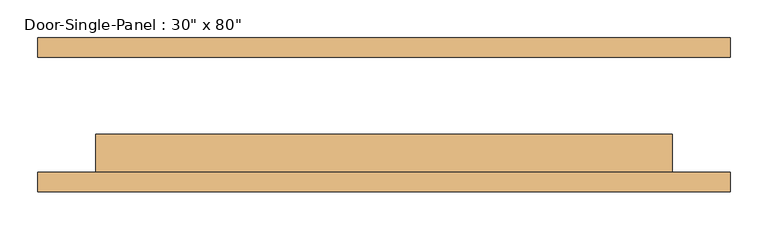
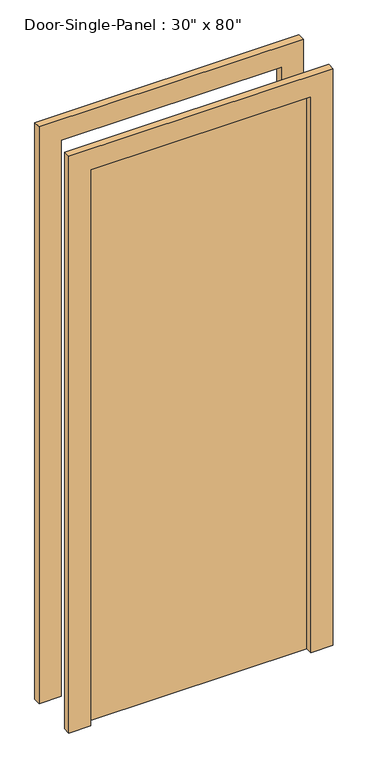
"""IFC4 building model written with IfcOpenShell, lengths in millimetres: door geometry."""

from ifc_helpers import new_model, si_unit, frame, origin, origin_with_axes, place, context, project, spatial, polyline, outline, extrude, source, transform, mapped, element, save


def door_d64d7266(model_context):
    return source(origin(), model_context, "Body", "SweptSolid", [
        extrude(outline(polyline([(381.0, -25.4), (381.0, -76.2), (-381.0, -76.2), (-381.0, -25.4), (381.0, -25.4)])), origin_with_axes(), (0.0, 0.0, 1.0), 2032.0),
        extrude(outline(polyline([(2108.2, -457.2), (0.0, -457.2), (0.0, -381.0), (2032.0, -381.0), (2032.0, 381.0), (0.0, 381.0), (0.0, 457.2), (2108.2, 457.2), (2108.2, -457.2)])), frame((0.0, -101.6, 0.0), z_axis=(0.0, 1.0, 0.0), x_axis=(0.0, 0.0, 1.0)), (0.0, 0.0, 1.0), 25.4),
        extrude(outline(polyline([(2108.2, 457.2), (2108.2, -457.2), (0.0, -457.2), (0.0, -381.0), (2032.0, -381.0), (2032.0, 381.0), (0.0, 381.0), (0.0, 457.2), (2108.2, 457.2)])), frame((0.0, 76.2, 0.0), z_axis=(0.0, 1.0, 0.0), x_axis=(0.0, 0.0, 1.0)), (0.0, 0.0, 1.0), 25.4),
    ])


if __name__ == "__main__":
    model = new_model("IFC4")
    model_context = context("Model", 3, world=origin())
    ifc_project = project(units=[si_unit("LENGTHUNIT", "METRE", prefix="MILLI")], contexts=[model_context])
    site = spatial("IfcSite", under=ifc_project)
    building = spatial("IfcBuilding", under=site)
    placement = place(None, origin())
    door_shape = door_d64d7266(model_context)
    element("IfcDoor", 1, ObjectType="Door-Single-Panel : 30\" x 80\"", at=placement, inside=building, context=model_context, shape_type="MappedRepresentation", body=[
        mapped(door_shape, transform((0.0, 0.0, 0.0), x_axis=(1.0, 0.0, 0.0), y_axis=(0.0, 1.0, 0.0), z_axis=(0.0, 0.0, 1.0))),
    ])
    save(model, "model.ifc")

# Revit data of these elements
# Type "Door-Single-Panel : 30\" x 80\""
#   Type Mark = "11"
#   Construction Type Id = "DOOR"
#   Assembly Code = "C1020300"
#   Analytic Construction = "Wooden"
#   Thickness = 0' - 2"
#   Thermal Resistance (R) = 2.5876 (h·ft²·°F)/BTU
#   Swing Angle [instance default] = 90.00°
#   Heat Transfer Coefficient (U) = 0.3865 BTU/(h·ft²·°F)
#   Height = 6' - 8"
#   Trim Projection Ext = 0' - 1"
#   Trim Projection Int = 0' - 1"
#   Trim Width = 0' - 3"
#   Width = 2' - 6"
#   Define Thermal Properties by = 1
#   Panel Material = Wood - Birch - Solid Stained Light Low Gloss
#   Trim Material = Paint - Sienna
#   Visual Light Transmittance = 0
#   Solar Heat Gain Coefficient = 0
#   Function = (empty or 0)
#   Wall Closure = (empty or 0)
# Element 1 (IfcDoor, "Door-Single-Panel : 30\" x 80\"")
#   Materials on its faces: "Paint - Sienna", "Wood - Birch - Solid Stained Light Low Gloss"
# Materials
#   "Wood - Birch - Solid Stained Light Low Gloss": class "Wood", colour RGB 210 159 95, transparency 0, Cost = 0
#   "Paint - Sienna": colour RGB 118 70 51, transparency 0, Cost = 0
